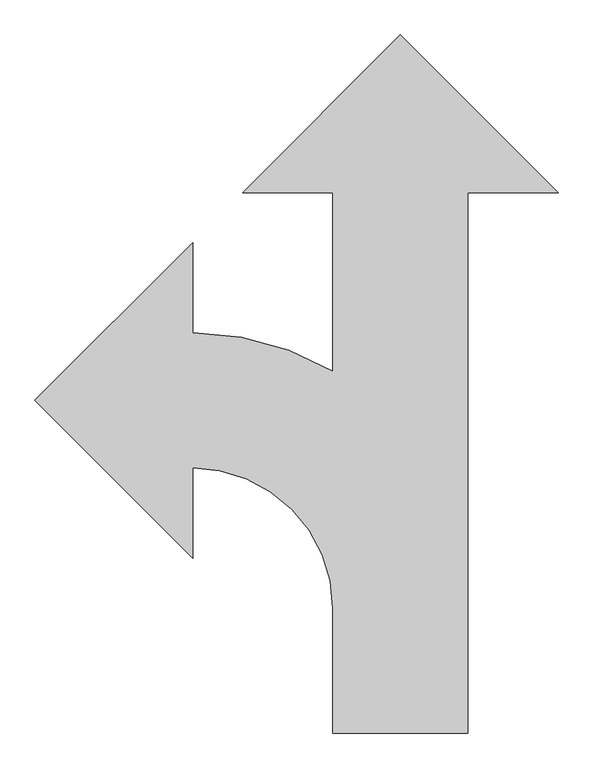
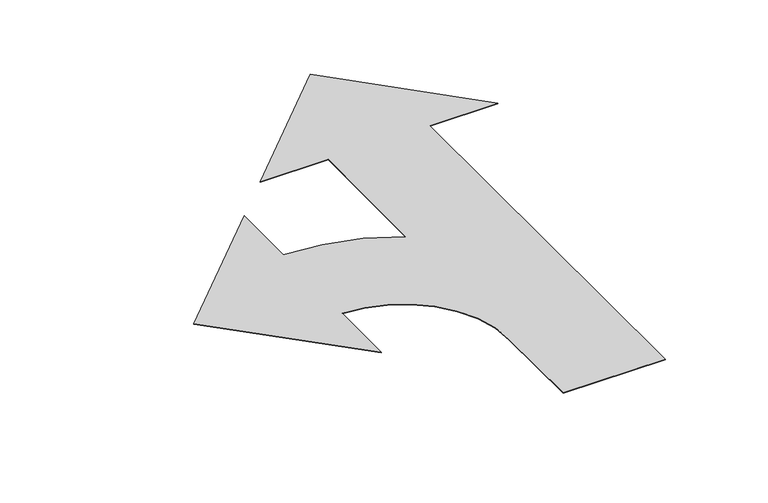
"""IFC4 building model written with IfcOpenShell, lengths in millimetres: geographic element geometry."""

from ifc_helpers import new_model, si_unit, point, frame_2d, origin, origin_with_axes, place, context, project, spatial, polyline, circle_curve, trimmed, segment, composite_curve, outline, extrude, source, transform, mapped, element, save


def geographic_element_33b6fea6(model_context):
    return source(origin(), model_context, "Body", "SweptSolid", [
        extrude(outline(composite_curve([segment(polyline([(0.0, 1574.8), (355.6, 1219.2), (152.4, 1219.2), (152.4, 0.0), (-152.4, 0.0), (-152.4, 281.6431186)]), True, "CONTINUOUS"), segment(trimmed(circle_curve(frame_2d((-468.7784407, 281.6431186)), 316.3784407), [point((-152.4, 281.6431186))], [point((-468.7784407, 598.0215593))], True, "CARTESIAN"), True, "CONTINUOUS"), segment(polyline([(-468.7784407, 598.0215593), (-468.7784407, 394.8215593), (-824.3784407, 750.4215593), (-468.7784407, 1106.0215593), (-468.7784407, 902.8215593)]), True, "CONTINUOUS"), segment(trimmed(circle_curve(frame_2d((-468.7784407, 281.6431186)), 621.1784407), [point((-468.7784407, 902.8215593))], [point((-152.4, 816.2152255))], False, "CARTESIAN"), True, "CONTINUOUS"), segment(polyline([(-152.4, 816.2152255), (-152.4, 1219.2), (-355.6, 1219.2), (0.0, 1574.8)]), True, "CONTINUOUS")], self_intersect=False)), origin_with_axes(), (0.0, 0.0, 1.0), 1.5875),
    ])


if __name__ == "__main__":
    model = new_model("IFC4")
    model_context = context("Model", 3, world=origin())
    ifc_project = project(units=[si_unit("LENGTHUNIT", "METRE", prefix="MILLI")], contexts=[model_context])
    site = spatial("IfcSite", under=ifc_project)
    building = spatial("IfcBuilding", under=site)
    placement = place(None, origin())
    geographic_element_shape = geographic_element_33b6fea6(model_context)
    element("IfcGeographicElement", 1, at=placement, inside=building, context=model_context, shape_type="MappedRepresentation", body=[
        mapped(geographic_element_shape, transform((0.0, 0.0, 0.0), x_axis=(1.0, 0.0, 0.0), y_axis=(0.0, 1.0, 0.0), z_axis=(0.0, 0.0, 1.0))),
    ])
    save(model, "model.ifc")

# Revit data of these elements
# Element 1 (IfcGeographicElement)
#   Materials on its faces: "Paint - White"
# Materials
#   "Paint - White": class "Paint", colour RGB 249 249 249, transparency 0
